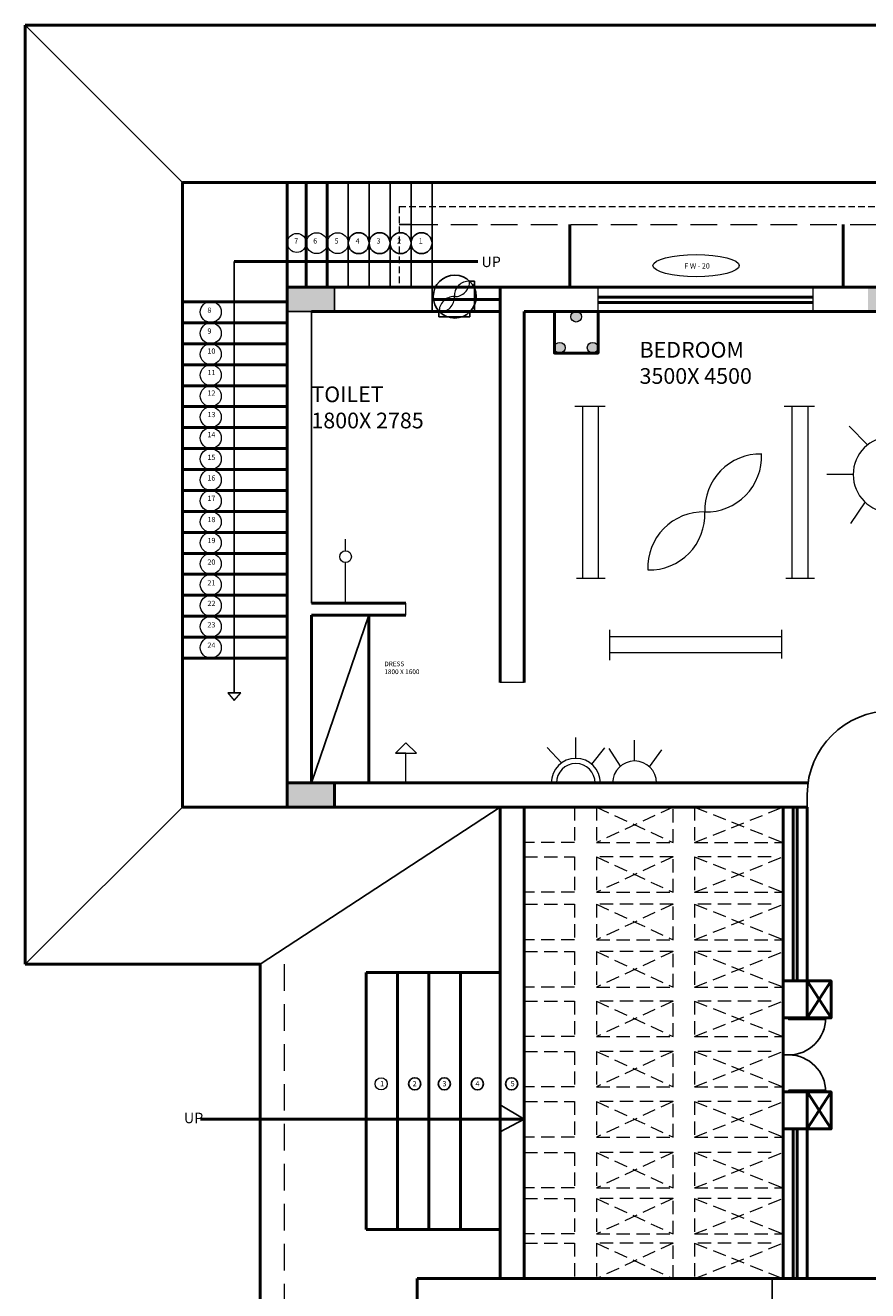
# Model space of a CAD drawing. Units: millimetres. Extents: x 15 to 330868, y -4710 to 1734924.
# Tile 3 of 3: x 309738 to 317776, y 856654 to 868729. Entities that reach past the tile are written whole.
import ezdxf

# ---------------------------------------------------------------- set-up
doc = ezdxf.new("R2010")
doc.units = ezdxf.units.MM
doc.header["$MEASUREMENT"] = 0
doc.linetypes.add('DASHED', pattern=[19.049999999999997, 12.7, -6.349999999999999])
for name, color, linetype, lineweight in [('A-ANNO-DIMS', 2, 'Continuous', 18), ('A-ANNO-TEXT', 7, 'Continuous', 18), ('A-AREA-IDEN', 30, 'Continuous', 25), ('A-COLS', 8, 'Continuous', 35), ('A-DOOR', 4, 'Continuous', 25), ('A-FLOR-OVHD', 8, 'DASHED', 18), ('A-FLOR-STRS', 3, 'Continuous', 25), ('A-ROOF', 6, 'Continuous', 25), ('A-ROOF-OVHD', 6, 'DASHED', 18), ('A-WALL', 7, 'Continuous', 50), ('E-LITE', 1, 'Continuous', 18)]:
    doc.layers.add(name, color=color, linetype=linetype, lineweight=lineweight)
doc.styles.get("Standard").update_dxf_attribs({"font": 'arial.ttf'})
doc.dimstyles.get("Standard").update_dxf_attribs({"dimtxt": 0.18, "dimasz": 0.18, "dimexe": 0.18, "dimexo": 0.0625, "dimgap": 0.09, "dimtad": 0, "dimtih": 1, "dimtoh": 1, "dimdec": 0, "dimzin": 0, "dimdsep": 46, "dimtxsty": 'Standard', "dimcen": 0.09, "dimadec": 0, "dimazin": 0, "dimtfac": 1, "dimtdec": 0, "dimtofl": 0, "dimtmove": 0, "dimatfit": 3, "dimfxl": 1, "dimtolj": 1, "dimtzin": 0, "dimarcsym": 0})

# ---------------------------------------------------------------- blocks, each defined once
blk = doc.blocks.new('*U5')
for p, q in [((0, 0), (-1e-16, -5.999999999999999)), ((40, -6e-16), (40, -6))]:
    blk.add_line(p, q)
blk.add_lwpolyline([(0, 0), (5.6e-15, 40), (1.750000000000007, 40), (1.749999999999998, -7e-16)], close=True)
blk.add_arc((0, 0), 40, 0, 90)
blk = doc.blocks.new('FAN-CEILING')
blk.add_line((543.2829999999958, 553.5), (543.2829999999958, 553.5))
for centre, radius, start, end in [((555.3863884535967, 1083.047616258962), 529.6859162592511, 268.5279151991481, 2.595751645517247), ((1072.491430036316, 575.9857168442104), 529.6859162592514, 88.52791519914813, 182.5957516455172), ((529.6754217544221, 23.98890125169419), 529.6859162592514, 88.52791519914813, 182.5957516455172), ((14.1405782456859, 529.5110987483058), 529.6859162592514, 268.5279151991481, 2.595751645517247)]:
    blk.add_arc(centre, radius, start, end)
blk = doc.blocks.new('FAN-EXHAUST')
blk.add_line((145.1339548087562, 148.0080506636295), (145.1339548087562, 148.0080506636295))
for centre, radius, start, end in [((148.3704525375506, 289.6113433190621), 141.6402746656115, 268.5279151991481, 2.595751652180509), ((286.6465476204758, 154.0208273150492), 141.6402746656116, 88.52791519914813, 182.5957516521805), ((141.4952303098398, 6.414522946579381), 141.6402746656116, 88.52791519914813, 182.5957516521805), ((3.639012893370818, 141.5933160863351), 141.6402746656116, 268.5279151991481, 2.595751652180509)]:
    blk.add_arc(centre, radius, start, end)
blk = doc.blocks.new('LIGHT-FTL')
for p, q in [((0, 289), (0, 0)), ((1640, 289), (1640, 15)), ((0, 224.5), (1640, 224.5)), ((0, 74.5), (1640, 74.5))]:
    blk.add_line(p, q)
blk = doc.blocks.new('*D17')
at = {"layer": 'A-ANNO-DIMS', "color": 0, "lineweight": -2, "transparency": 16777216}
for p, q in [((313978.3522373521, 866288.9542451887), (314023.1148893985, 866288.9542451887)), ((314022.9348893985, 866288.7742451887), (314022.9348893985, 866140.3201412783)), ((314022.9348893985, 865991.4998982135), (314022.9348893985, 866139.9540021241)), ((313978.3522373521, 865991.3198982136), (314023.1148893985, 865991.3198982136))]:
    blk.add_line(p, q, dxfattribs=at)
at = {"layer": 'A-ANNO-DIMS', "color": 0, "transparency": 16777216}
for points in [[(314022.9048893985, 866288.7742451887), (314022.9648893985, 866288.7742451887), (314022.9348893985, 866288.9542451887)], [(314022.9048893985, 865991.4998982135), (314022.9648893985, 865991.4998982135), (314022.9348893985, 865991.3198982136)]]:
    blk.add_solid(points, dxfattribs=at)
at = {"layer": 'Defpoints', "color": 0, "transparency": 16777216}
for p in [(313978.2897373521, 866288.9542451887), (314022.9348893985, 866288.9542451887), (313978.2897373521, 865991.3198982136)]:
    blk.add_point(p, dxfattribs=at)
at = {"layer": 'A-ANNO-DIMS', "color": 0, "transparency": 16777216, "insert": (314022.9348893987, 866140.1370717008), "char_height": 0.18, "attachment_point": 5}
blk.add_mtext('\\A1;EXHAUST FAN 298 TYP.', dxfattribs=at)
blk = doc.blocks.new('*D18')
at = {"layer": 'A-ANNO-DIMS', "color": 0, "lineweight": -2, "transparency": 16777216}
for p, q in [((313684.8639454954, 865991.2573982131), (313684.8639454954, 865946.4947461667)), ((313685.0439454954, 865946.6747461667), (313830.9772916283, 865946.6747461667)), ((313978.109737352, 865946.6747461667), (313832.176391219, 865946.6747461667)), ((313978.289737352, 865991.2573982131), (313978.289737352, 865946.4947461667))]:
    blk.add_line(p, q, dxfattribs=at)
at = {"layer": 'A-ANNO-DIMS', "color": 0, "transparency": 16777216}
for points in [[(313685.0439454954, 865946.7047461667), (313685.0439454954, 865946.6447461667), (313684.8639454954, 865946.6747461667)], [(313978.109737352, 865946.7047461667), (313978.109737352, 865946.6447461667), (313978.289737352, 865946.6747461667)]]:
    blk.add_solid(points, dxfattribs=at)
at = {"layer": 'Defpoints', "color": 0, "transparency": 16777216}
for p in [(313684.8639454954, 865991.3198982129), (313978.289737352, 865991.3198982129), (313978.289737352, 865946.6747461667)]:
    blk.add_point(p, dxfattribs=at)
at = {"layer": 'A-ANNO-DIMS', "color": 0, "transparency": 16777216, "insert": (313831.5768414237, 865946.6747461667), "char_height": 0.18, "attachment_point": 5}
blk.add_mtext('\\A1;293 TYP.', dxfattribs=at)

msp = doc.modelspace()

# ---------------------------------------------------------------- hatches: boundary and pattern name
at = {"layer": 'A-COLS'}
h = msp.add_hatch(color=256, dxfattribs=at)
h.dxf.hatch_style = 1
h.paths.add_polyline_path([(312687.5462042676, 861499.2884389247), (312237.5462042676, 861499.2884389247), (312237.5462042676, 861269.2884389245), (312687.5462042676, 861269.2884389245)])
h.paths.add_polyline_path([(312687.5462042676, 865999.2884389245), (312687.5462042676, 866229.2884389247), (312237.5462042676, 866229.2884389247), (312237.5462042676, 865999.2884389245)])
h.paths.add_polyline_path([(318227.5462042675, 866229.2884389248), (317777.5462042676, 866229.2884389248), (317777.5462042676, 865999.2884389247), (318227.5462042675, 865999.2884389247)])
h.paths.add_polyline_path([(321177.5462042676, 866229.2884389248), (321177.5462042676, 865999.2884389247), (321627.5462042676, 865999.2884389247), (321627.5462042676, 866229.2884389248)])
h.paths.add_polyline_path([(326187.5462042675, 866229.2884389248), (326187.5462042675, 865999.2884389247), (326637.5462042675, 865999.2884389247), (326637.5462042675, 866229.2884389248)])
h = msp.add_hatch(color=256, dxfattribs=at)
h.dxf.hatch_style = 1
h.paths.add_polyline_path([(314888.4257045456, 865653, 1), (314786.5742954544, 865653, 1)])
h.paths.add_polyline_path([(314943.5742954544, 865948.3627343792, 1), (315045.4257045456, 865948.3627343792, 1)])
h.paths.add_polyline_path([(315202.4257045456, 865652.9257045455, 1), (315100.5742954545, 865652.9257045455, 1)])

# ---------------------------------------------------------------- linework, layer by layer
at = {"layer": 'A-FLOR-OVHD', "ltscale": 10}
for p, q in [((315188.5, 861269.2884389245), (315918.5, 860930.5)), ((315918.5, 861269.2884389245), (315188.5, 860930.5)), ((315188.5, 860794.7884389245), (315918.5, 860456)), ((315918.5, 860794.7884389245), (315188.5, 860456)), ((315188.5, 860342.2884389244), (315918.5, 860003.5)), ((315918.5, 860342.2884389244), (315188.5, 860003.5)), ((315188.5, 859889.4999999998), (315918.5, 859550.7115610756)), ((315918.5, 859889.4999999998), (315188.5, 859550.7115610756)), ((315188.5, 859417.9999999999), (315918.5, 859079.2115610755)), ((315918.5, 859417.9999999999), (315188.5, 859079.2115610755)), ((315188.5, 858938), (315918.5, 858599.2115610755)), ((315918.5, 858938), (315188.5, 858599.2115610755)), ((315188.5, 858458.9999999998), (315918.5, 858120.2115610755)), ((315918.5, 858458.9999999998), (315188.5, 858120.2115610755)), ((315188.5, 857973.4999999999), (315918.5, 857634.7115610754)), ((315918.5, 857973.4999999999), (315188.5, 857634.7115610754)), ((315188.5000000001, 857534.2884389247), (315918.5000000001, 857195.5)), ((315918.5000000001, 857534.2884389247), (315188.5000000001, 857195.5)), ((315188.5000000002, 857108.076877849), (315918.5000000001, 856769.2884389245)), ((315918.5000000001, 857108.076877849), (315188.5000000002, 856769.2884389245))]:
    msp.add_line(p, q, dxfattribs=at)
for points in [[(314497.5462042676, 861269.2884389245), (314977, 861269.2884389245), (314977, 860930.5), (314497.5462042676, 860930.5)], [(315188.5, 860930.5), (315918.5, 860930.5), (315918.5, 861269.2884389245), (315188.5, 861269.2884389245)], [(314497.5462042676, 860794.7884389245), (314977, 860794.7884389245), (314977, 860456), (314497.5462042676, 860456)], [(315188.5, 860456), (315918.5, 860456), (315918.5, 860794.7884389245), (315188.5, 860794.7884389245)], [(314497.5462042676, 860342.2884389246), (314977, 860342.2884389246), (314977, 860003.5), (314497.5462042676, 860003.5)], [(315188.5, 860003.5), (315918.5, 860003.5), (315918.5, 860342.2884389244), (315188.5, 860342.2884389244)], [(314497.5462042676, 859889.5), (314977, 859889.5), (314977, 859550.7115610756), (314497.5462042676, 859550.7115610756)], [(315188.5, 859550.7115610756), (315918.5, 859550.7115610756), (315918.5, 859889.4999999998), (315188.5, 859889.4999999998)], [(314497.5462042676, 859418), (314977, 859418), (314977, 859079.2115610755), (314497.5462042676, 859079.2115610755)], [(315188.5, 859079.2115610755), (315918.5, 859079.2115610755), (315918.5, 859417.9999999999), (315188.5, 859417.9999999999)], [(314497.5462042676, 858938), (314977, 858938), (314977, 858599.2115610755), (314497.5462042676, 858599.2115610755)], [(315188.5, 858599.2115610755), (315918.5, 858599.2115610755), (315918.5, 858938), (315188.5, 858938)], [(314497.5462042676, 858459), (314977, 858459), (314977, 858120.2115610755), (314497.5462042676, 858120.2115610755)], [(315188.5, 858120.2115610755), (315918.5, 858120.2115610755), (315918.5, 858458.9999999998), (315188.5, 858458.9999999998)], [(314497.5462042676, 857973.5000000001), (314977, 857973.5000000001), (314977, 857634.7115610754), (314497.5462042676, 857634.7115610754)], [(315188.5, 857634.7115610754), (315918.5, 857634.7115610754), (315918.5, 857973.4999999999), (315188.5, 857973.4999999999)], [(314497.5462042676, 857534.2884389248), (314977.0000000001, 857534.2884389248), (314977.0000000001, 857195.5), (314497.5462042676, 857195.5)], [(315188.5000000001, 857195.5), (315918.5000000001, 857195.5), (315918.5000000001, 857534.2884389247), (315188.5000000001, 857534.2884389247)], [(314497.5462042677, 857108.0768778491), (314977.0000000001, 857108.0768778491), (314977.0000000001, 856769.2884389245), (314497.5462042677, 856769.2884389245)], [(315188.5000000002, 856769.2884389245), (315918.5000000001, 856769.2884389245), (315918.5000000001, 857108.076877849), (315188.5000000002, 857108.076877849)]]:
    msp.add_lwpolyline(points, close=True, dxfattribs=at)
at = {"layer": 'A-FLOR-STRS'}
for p, q in [((312818.5, 866229.2884389247), (312818.5, 867229.2884389246)), ((313018.5, 866229.2884389247), (313018.5, 867229.2884389246)), ((313218.5, 866229.2884389247), (313218.5, 867229.2884389246)), ((313418.5, 866229.2884389247), (313418.5, 867229.2884389246)), ((313618.5, 866229.2884389247), (313618.5, 867229.2884389246)), ((313418.5, 866829.2884389249), (313305, 866829.2884389249)), ((311732, 866476.5), (311732, 862359)), ((313618.5, 865999.2884389247), (313618.5, 866229.2884389247)), ((312467.5462042676, 865999.2884389247), (312467.5462042676, 863214.2884389246)), ((311732, 862359), (311670, 862359)), ((311670, 862359), (311794, 862359)), ((311794, 862359), (311670, 862359)), ((311794, 862359), (311732, 862359)), ((314497.5462042675, 858289.6057805378), (314267.5462042676, 858426.5)), ((314497.5462042676, 858289.6057805378), (314267.5462042676, 858170.5000000001)), ((314267.5462042676, 857239.5), (314267.5462042676, 857239.5))]:
    msp.add_line(p, q, dxfattribs=at)
msp.add_lwpolyline([(312687.5462042676, 866229.2884389247), (312687.5462042676, 865999.2884389245), (312237.5462042676, 865999.2884389245), (312237.5462042676, 866229.2884389247)], close=True, dxfattribs=at)
for centre, radius in [((312918.5, 866650.5), 100), ((313118.5, 866650.5), 100), ((313318.5, 866650.5), 100), ((313518.5, 866650.5), 100), ((313835.0144525376, 866140.3010686532), 204.7952742509166), ((313453.5, 858628), 58), ((313736, 858628), 58), ((314051.5000000001, 858628), 58), ((314378, 858628), 58)]:
    msp.add_circle(centre, radius, dxfattribs=at)
at = {"layer": 'A-ROOF'}
for p, q in [((309737.5462042676, 868729.2884389249), (311237.5462042676, 867229.2884389248)), ((312467.5462042675, 861499.2884389247), (313016, 863099.2884389247)), ((309737.5462042676, 859769.2884389244), (311237.5462042676, 861269.2884389245)), ((311977.5000000001, 859769.2884389248), (314267.5462042676, 861269.2884389245))]:
    msp.add_line(p, q, dxfattribs=at)
at = {"layer": 'A-ROOF-OVHD', "ltscale": 5}
for p, q in [((313305.0000000001, 866999.288438925), (329137.5462042676, 866999.2884389248)), ((313305, 866999.288438925), (313305, 866229.2884389247))]:
    msp.add_line(p, q, dxfattribs=at)
at = {"layer": 'A-ROOF-OVHD', "ltscale": 20}
for p, q in [((313418.5, 866829.2884389249), (327915, 866829.2884389247)), ((312207.5000000001, 859769.2884389248), (312207.5000000001, 848959.2884389246))]:
    msp.add_line(p, q, dxfattribs=at)
at = {"layer": 'A-ROOF-OVHD', "ltscale": 10}
for p, q in [((316123.5, 860930.4999999999), (316969.2049794545, 861269.2884389245)), ((316123.5, 861269.2884389245), (316969.2049794545, 860930.4999999999)), ((316123.5, 860455.9999999999), (316969.2049794545, 860794.7884389245)), ((316123.5, 860794.7884389245), (316969.2049794545, 860455.9999999999)), ((316123.5, 860003.5), (316969.2049794545, 860342.2884389244)), ((316123.5, 860342.2884389244), (316969.2049794545, 860003.5)), ((316123.5, 859550.7115610754), (316969.2049794545, 859889.4999999998)), ((316123.5, 859889.4999999997), (316969.2049794545, 859550.7115610754)), ((316123.5, 859079.2115610753), (316969.2049794545, 859417.9999999999)), ((316123.5, 859417.9999999999), (316969.2049794545, 859079.2115610753)), ((316123.5, 858599.2115610753), (316969.2049794545, 858938)), ((316123.5, 858937.9999999998), (316969.2049794545, 858599.2115610753)), ((316123.5, 858120.2115610754), (316969.2049794545, 858458.9999999998)), ((316123.5, 858458.9999999998), (316969.2049794545, 858120.2115610754)), ((316123.5, 857634.7115610753), (316969.2049794545, 857973.4999999999)), ((316123.5, 857973.4999999997), (316969.2049794545, 857634.7115610753)), ((316123.5000000001, 857195.5), (316969.2049794545, 857534.2884389247)), ((316123.5000000001, 857534.2884389245), (316969.2049794545, 857195.5)), ((316123.5000000001, 856769.2884389244), (316969.2049794546, 857108.076877849)), ((316123.5000000001, 857108.076877849), (316969.2049794546, 856769.2884389244))]:
    msp.add_line(p, q, dxfattribs=at)
for points in [[(316853.5, 861269.2884389245), (316123.5, 861269.2884389245), (316123.5, 860930.4999999999), (316969.2049794545, 860930.4999999999)], [(316853.5, 860794.7884389245), (316123.5, 860794.7884389245), (316123.5, 860455.9999999999), (316969.2049794545, 860455.9999999999)], [(316853.5, 860342.2884389244), (316123.5, 860342.2884389244), (316123.5, 860003.5), (316969.2049794545, 860003.5)], [(316853.5, 859889.4999999997), (316123.5, 859889.4999999997), (316123.5, 859550.7115610754), (316969.2049794545, 859550.7115610754)], [(316853.5, 859417.9999999999), (316123.5, 859417.9999999999), (316123.5, 859079.2115610753), (316969.2049794545, 859079.2115610753)], [(316853.5, 858937.9999999998), (316123.5, 858937.9999999998), (316123.5, 858599.2115610753), (316969.2049794545, 858599.2115610753)], [(316853.5, 858458.9999999998), (316123.5, 858458.9999999998), (316123.5, 858120.2115610754), (316969.2049794545, 858120.2115610754)], [(316853.5, 857973.4999999997), (316123.5, 857973.4999999997), (316123.5, 857634.7115610753), (316969.2049794545, 857634.7115610753)], [(316853.5000000001, 857534.2884389245), (316123.5000000001, 857534.2884389245), (316123.5000000001, 857195.5), (316969.2049794545, 857195.5)], [(316853.5000000002, 857108.076877849), (316123.5000000001, 857108.076877849), (316123.5000000001, 856769.2884389244), (316969.2049794546, 856769.2884389244)]]:
    msp.add_lwpolyline(points, dxfattribs=at)
at = {"layer": 'A-WALL'}
for p, q in [((309737.5462042676, 868729.2884389249), (309737.5462042676, 859769.2884389246)), ((309737.5462042676, 868729.2884389249), (319602.7731021338, 868729.2884389249)), ((311237.5462042676, 867229.2884389248), (329367.5462042676, 867229.2884389248)), ((311237.5462042676, 867229.2884389246), (311237.5462042676, 861269.2884389245)), ((312237.5462042676, 867229.2884389246), (312237.5462042676, 861269.2884389245)), ((312418.5000000001, 866229.2884389247), (312418.5, 867229.2884389246)), ((312618.5, 866229.2884389247), (312618.4999999999, 867229.2884389246)), ((314932.5, 866229.2884389247), (314932.5, 866829.2884389247)), ((317541, 866229.2884389247), (317541.0000000001, 866829.2884389247)), ((314057, 866476.5), (311732, 866476.5)), ((312237.5462042676, 866229.2884389247), (314267.5462042676, 866229.2884389247)), ((314267.5462042676, 866229.2884389247), (314267.5462042676, 862457.5)), ((314267.5462042676, 866229.2884389247), (320317.5462042675, 866229.2884389248)), ((312237.5462042676, 866090.5000000001), (311237.5462042676, 866090.5000000001)), ((313618.5, 866114.2884389247), (314267.5462042676, 866114.2884389247)), ((315202.5, 866134.2884389247), (317253.5, 866134.2884389247)), ((315202.5, 866084.2884389246), (317253.5, 866084.2884389246)), ((312467.5462042676, 865999.2884389245), (314267.5462042676, 865999.2884389245)), ((314497.5462042676, 865999.2884389248), (314497.5462042675, 862457.5)), ((314497.5462042676, 865999.2884389247), (320317.5462042676, 865999.2884389248)), ((312237.5462042676, 865890.5000000002), (311237.5462042676, 865890.5000000002)), ((312237.5462042676, 865690.5000000001), (311237.5462042676, 865690.5000000001)), ((312237.5462042676, 865490.5000000002), (311237.5462042676, 865490.5000000002)), ((312237.5462042676, 865290.5000000002), (311237.5462042676, 865290.5000000002)), ((312237.5462042676, 865090.5000000001), (311237.5462042676, 865090.5000000001)), ((312237.5462042676, 864890.5000000002), (311237.5462042676, 864890.5000000002)), ((312237.5462042676, 864690.5000000002), (311237.5462042676, 864690.5000000002)), ((312237.5462042676, 864490.5000000001), (311237.5462042676, 864490.5000000001)), ((312237.5462042676, 864290.5000000002), (311237.5462042676, 864290.5000000002)), ((312237.5462042676, 864090.5000000001), (311237.5462042676, 864090.5000000001)), ((312237.5462042676, 863890.5000000001), (311237.5462042676, 863890.5000000001)), ((312237.5462042676, 863690.5000000002), (311237.5462042676, 863690.5000000002)), ((312237.5462042676, 863490.5000000001), (311237.5462042676, 863490.5000000001)), ((312237.5462042676, 863290.5), (311237.5462042676, 863290.5)), ((312467.5462042676, 863214.2884389246), (313367.5462042675, 863214.2884389246)), ((312237.5462042676, 863090.5000000002), (311237.5462042676, 863090.5000000002)), ((312467.5462042676, 863099.2884389247), (313367.5462042675, 863099.2884389247)), ((312467.5462042676, 863099.2884389247), (312467.5462042675, 861499.2884389247)), ((313016, 863099.2884389247), (313016, 861499.2884389247)), ((312237.5462042676, 862890.5000000001), (311237.5462042676, 862890.5000000001)), ((312237.5462042676, 862690.5000000002), (311237.5462042676, 862690.5000000002)), ((312467.5462042675, 861499.2884389247), (317206.8541594452, 861499.2884389247)), ((311237.5462042676, 861269.2884389247), (317199.2049794545, 861269.2884389245)), ((314267.5462042676, 861269.2884389247), (314267.5462042676, 856769.2884389245)), ((314497.5462042676, 861269.2884389245), (314497.5462042675, 856769.2884389245)), ((316969.2049794545, 861269.2884389245), (316969.2049794545, 856769.2884389247)), ((317064.2049794545, 859611), (317064.2049794546, 861269.2884389245)), ((317104.2049794545, 859611), (317104.2049794546, 861269.2884389245)), ((317199.2049794545, 861269.2884389245), (317199.2049794545, 859257.053530784)), ((309737.5462042675, 859769.2884389244), (311977.5000000001, 859769.2884389248)), ((311977.5000000001, 859769.2884389248), (311977.5000000001, 848729.2884389246)), ((314267.5462042676, 859691.0000000001), (312989.5, 859691.0000000001)), ((312989.5, 859691.0000000001), (312989.5, 857239.5)), ((313289.5, 859691.0000000001), (313289.5, 857239.5)), ((313589.5, 859691.0000000001), (313589.5, 857239.5)), ((313889.5, 859691.0000000001), (313889.5, 857239.5)), ((316969.2049794545, 859611), (316969.2049794545, 858197.5768778491)), ((317199.2049794545, 859257.053530784), (317426.158775187, 859611)), ((317199.2049794544, 859611), (317426.158775187, 859257.053530784)), ((317199.2049794545, 858197.5768778491), (317426.158775187, 858551.5233470649)), ((317199.2049794544, 858551.5233470649), (317426.158775187, 858197.5768778491)), ((317199.2049794545, 858551.5233470651), (317199.2049794545, 856769.2884389245)), ((314497.5462042676, 858289.6057805378), (311410, 858289.6057805378)), ((317064.2049794545, 858197.5768778491), (317064.2049794545, 856769.2884389247)), ((317104.2049794545, 858197.5768778491), (317104.2049794545, 856769.2884389247)), ((312989.5, 857239.5), (314267.5462042676, 857239.5)), ((313477.5, 856769.2884389245), (321177.5462042676, 856769.2884389247)), ((313477.5, 856769.2884389245), (313477.5, 856087))]:
    msp.add_line(p, q, dxfattribs=at)
for points in [[(315202.5, 865999.2884389247), (314786.5, 865999.2884389247), (314786.5, 865602), (315202.5, 865602)], [(312687.5462042676, 861499.2884389247), (312687.5462042676, 861269.2884389245), (312237.5462042676, 861269.2884389245), (312237.5462042676, 861499.2884389247)], [(316969.2049794546, 859257.053530784), (317199.2049794544, 859257.053530784), (317199.2049794544, 859611), (316969.2049794546, 859611)], [(317199.2049794544, 859611), (317426.158775187, 859611), (317426.158775187, 859257.053530784), (317199.2049794544, 859257.053530784)], [(316969.2049794546, 858197.5768778491), (317199.2049794544, 858197.5768778491), (317199.2049794544, 858551.5233470649), (316969.2049794546, 858551.5233470649)], [(317199.2049794544, 858551.5233470649), (317426.158775187, 858551.5233470649), (317426.158775187, 858197.5768778491), (317199.2049794544, 858197.5768778491)]]:
    msp.add_lwpolyline(points, close=True, dxfattribs=at)
for points in [[(316969.2049794545, 856769.2884389244), (316969.2049794545, 856989.2884389245)], [(317199.2049794545, 856989.2884389245), (317199.2049794545, 856769.2884389245)]]:
    msp.add_lwpolyline(points, dxfattribs=at)
at = {"layer": 'E-LITE'}
for p, q in [((315202.5, 865999.2884389247), (315202.5, 866229.2884389247)), ((317253.5, 866229.2884389247), (317253.5, 865999.2884389247)), ((317774.193618227, 864724.3873621623), (317599.987389306, 864903.6976792249)), ((317637.5059287428, 864442), (317387.5059287428, 864442)), ((317752.5, 864182.5), (317612.4294522584, 863975.4245508147)), ((312793.5, 863714.5000000002), (312793.5, 863827)), ((312793.5, 863214.2884389246), (312793.5, 863602.5000000001)), ((313367.5462042676, 863099.2884389247), (313367.5462042676, 863214.2884389246)), ((314497.5462042676, 862457.5), (314267.5462042676, 862457.5)), ((311670, 862359), (311732, 862286.5)), ((311732, 862286.5), (311794, 862359)), ((314990.5, 861734.2884389247), (314990.5, 861934.2884389245)), ((313369, 861883.5), (313269, 861783.5000000001)), ((313269, 861783.5000000001), (313369, 861883.5)), ((313369, 861883.5), (313469, 861783.4999999999)), ((314853.6841582928, 861690.354986122), (314717.6042632716, 861836.9232711327)), ((315143.7394902659, 861677.4531341454), (315268.7997110762, 861833.5298498042)), ((315416.4617291272, 861660.1133915896), (315310.2806171569, 861829.5995900268)), ((315551.5, 861709.2884389247), (315551.5, 861909.2884389246)), ((315694.5678242209, 861653.0141611468), (315810.3641397665, 861816.082285886)), ((313369, 861783.5000000001), (313269, 861783.5000000001)), ((313269, 861783.5000000001), (313369, 861783.4999999999)), ((313369, 861499.2884389247), (313369, 861783.5000000001)), ((313369, 861783.4999999999), (313469, 861783.4999999999)), ((313224.5, 861499.2884389247), (313369, 861499.2884389247)), ((317199.2049794545, 859611), (317199.2049794545, 859257.053530784)), ((317199.2049794545, 858551.5233470651), (317199.2049794545, 858197.5768778491))]:
    msp.add_line(p, q, dxfattribs=at)
for centre, radius in [((312518.5, 866650.5), 100), ((312718.5, 866650.5), 100), ((312328.0231021338, 866652.5000000001), 90.47689786623232), ((311507.5462042673, 865993.5), 100), ((314994.5000000001, 865948.3627343792), 50.92570454556905), ((311507.5462042673, 865790.5000000001), 100), ((311507.5462042673, 865590.5), 100), ((314837.5, 865653), 50.92570454556905), ((315151.5, 865652.9257045455), 50.92570454556905), ((311507.5462042673, 865390.4999999999), 100), ((311507.5462042674, 865190.5000000001), 100), ((311507.5462042674, 864990.5000000002), 100), ((311507.5462042674, 864790.4999999999), 100), ((311507.5462042674, 864590.5), 100), ((311507.5462042674, 864390.5000000001), 100), ((311507.5462042674, 864190.4999999999), 100), ((311507.5462042674, 863990.5), 100), ((311507.5462042674, 863790.5000000001), 100), ((311507.5462042674, 863590.5000000001), 100), ((312793.5, 863658.5000000001), 56), ((311507.5462042674, 863390.5), 100), ((311507.5462042674, 863190.5000000001), 100), ((311507.5462042676, 862990.5), 100), ((311507.5462042676, 862790.5), 100), ((313133.5, 858628), 58)]:
    msp.add_circle(centre, radius, dxfattribs=at)
for centre, radius, start, end in [((317997.5462042676, 864442), 360.0402755247991, 90, 270), ((314990.5, 861499.2884389247), 235, 0, 180), ((314990.5, 861499.2884389247), 185, 0, 180), ((315551.5, 861499.2884389247), 210, 0, 180)]:
    msp.add_arc(centre, radius, start, end, dxfattribs=at)
msp.add_ellipse((316139, 866436.5000000001), major_axis=(411.9999999999999, 0), ratio=0.2572815533980583, dxfattribs=at)

# ---------------------------------------------------------------- block references
at = {"layer": 'A-DOOR', "xscale": -19.95853062032723, "yscale": 19.95853062032723, "zscale": 19.95853062032723}
msp.add_blockref('*U5', (317997.5462042675, 861389.0396226466), dxfattribs=at)
at = {"layer": 'A-DOOR'}
for p, xscale, yscale, zscale, rotation in [((317022.1197432335, 859257.053530784), 8.819127296487046, 8.819127296487046, 8.819127296487046, 270), ((317022.1197432335, 858551.5233470651), -8.819127296487046, 8.819127296487046, 8.819127296487046, 270), ((317907.5, 856612.6702075743), 26.10303855837779, 26.10303855837779, 26.10303855837779, 180)]:
    msp.add_blockref('*U5', p, dxfattribs=dict(at, xscale=xscale, yscale=yscale, zscale=zscale, rotation=rotation))
at = {"layer": 'E-LITE'}
for name, p in [('FAN-EXHAUST', (313686.644, 865992.33)), ('FAN-CEILING', (315678.467, 863532)), ('LIGHT-FTL', (315312.5, 862671))]:
    msp.add_blockref(name, p, dxfattribs=at)
at = {"layer": 'E-LITE', "rotation": 270}
for p in [(314981, 865090.4999999999), (316979, 865090.4999999999)]:
    msp.add_blockref('LIGHT-FTL', p, dxfattribs=at)

# ---------------------------------------------------------------- texts
at = {"layer": 'A-ANNO-TEXT', "attachment_point": 1}
for s, width, insert, char_height in [('7', 4478, (312303.5, 866696.5000000002), 50), ('6', 4478, (312485, 866696.5000000002), 50), ('5', 4478, (312688.5, 866696.5000000002), 50), ('4', 4478, (312890, 866696.5000000002), 50), ('3', 4478, (313089.5000000001, 866696.5000000002), 50), ('2', 4478, (313285.5, 866696.5000000002), 50), ('1', 4478, (313491.5, 866696.5000000002), 50), ('UP', 4478, (314090.5, 866522.2053206003), 100), ('F W - 20', 696.4999999999999, (316026.5, 866458.2387448841), 50), ('8', 4478, (311475.5462042673, 866035.5), 50), ('9', 4478, (311475.5462042673, 865837), 50), ('10', 4478, (311475.5462042673, 865645.5000000001), 50), ('11', 4478, (311475.5462042673, 865441.5), 50), ('12', 4478, (311475.5462042673, 865244.5), 50), ('13', 4478, (311475.5462042673, 865040), 50), ('14', 4478, (311475.5462042673, 864847.5000000001), 50), ('15', 4478, (311475.5462042673, 864631.4999999999), 50), ('16', 4478, (311475.5462042673, 864434.4999999999), 50), ('17', 4478, (311475.5462042673, 864240), 50), ('18', 4478, (311475.5462042673, 864038), 50), ('19', 4478, (311475.5462042673, 863838), 50), ('20', 4478, (311475.5462042673, 863632), 50), ('21', 4478, (311475.5462042673, 863434), 50), ('22', 4478, (311475.5462042673, 863238), 50), ('23', 4478, (311475.5462042673, 863033.5), 50), ('24', 4478, (311475.5462042673, 862839), 50), ('1', 4478, (313123.5, 858654.5), 50), ('2', 4478, (313434, 858654.5), 50), ('3', 4478, (313719, 858654.5), 50), ('4', 4478, (314033, 858654.5), 50), ('5', 4478, (314369.5000000001, 858654.5), 50), ('UP', 4478, (311251, 858352.7046384721), 100)]:
    msp.add_mtext_dynamic_manual_height_columns(s, width=width, gutter_width=1, heights=[0], dxfattribs=dict(at, insert=insert, char_height=char_height))
at = {"layer": 'A-AREA-IDEN', "char_height": 150, "attachment_point": 1}
for s, insert in [('BEDROOM\\P3500X 4500', (315599.0462042675, 865708)), ('TOILET\\P1800X 2785', (312467.5462042676, 865283.1754330128)), ('{\\H0.3x;DRESS\\P1800 X 1600}', (313163.5, 862658))]:
    msp.add_mtext_dynamic_manual_height_columns(s, width=7683.453795732522, gutter_width=1, heights=[0], dxfattribs=dict(at, insert=insert))

# ---------------------------------------------------------------- dimensions: what is measured, and where the dimension line sits
at = {"layer": 'A-ANNO-DIMS'}
dim = msp.add_linear_dim(base=(314022.9348893985, 866288.9542451887), p1=(313978.289737352, 865991.3198982129), p2=(313978.289737352, 866288.9542451884), angle=90, text='EXHAUST FAN <> TYP.', dimstyle='Standard', override={"dimdec": 0, "dimlfac": 1, "dimrnd": 0, "dimzin": 0, "dimdsep": 46, "dimlunit": 2}, dxfattribs=at)
dim.commit()
dim.dimension.update_dxf_attribs({"geometry": '*D17', "text_midpoint": (314022.9348893987, 866140.1370717008)})
dim = msp.add_linear_dim(base=(313978.289737352, 865946.6747461667), p1=(313684.8639454954, 865991.3198982129), p2=(313978.289737352, 865991.3198982129), text='<> TYP.', dimstyle='Standard', override={"dimdec": 0, "dimlfac": 1, "dimrnd": 0, "dimzin": 0, "dimdsep": 46, "dimlunit": 2}, dxfattribs=at)
dim.commit()
dim.dimension.update_dxf_attribs({"geometry": '*D18', "text_midpoint": (313831.5768414237, 865946.6747461667)})

doc.saveas('drawing.dxf')
